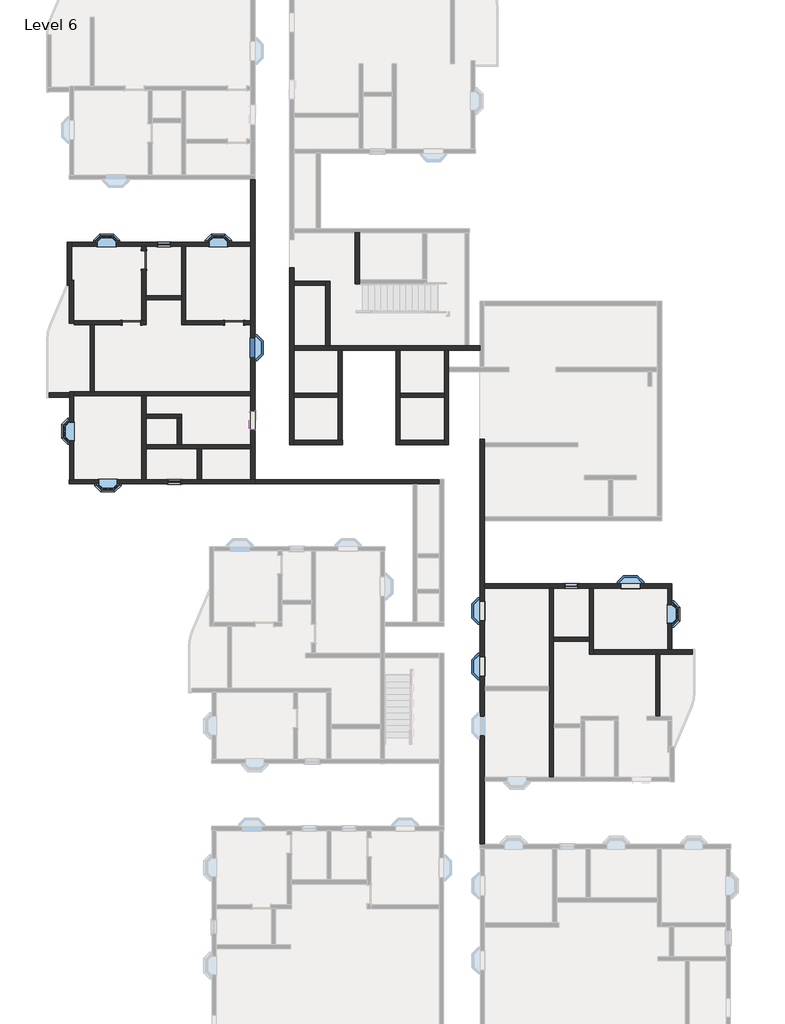
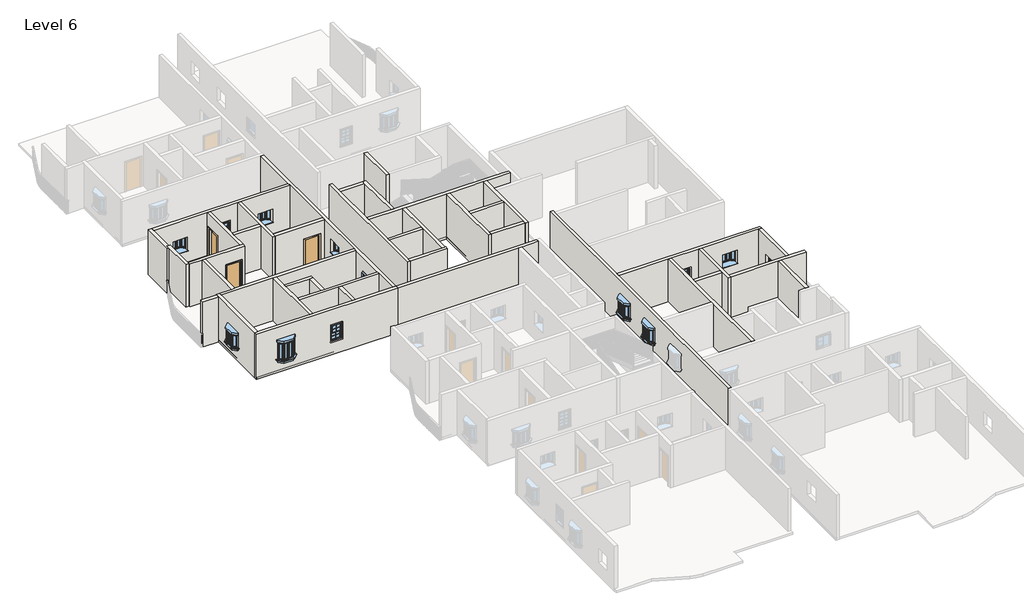
# One storey, part 3 of 14: 40 walls, 13 windows, 3 doors.
# Revit data of these elements (continued)
# Element 26 (IfcWall, "9\"")
#   Top Offset = 0' - 0"
#   Base Offset = 0' - 0"
#   wall height = 10' - 0"
#   Phase Created = New Construction
#   Base Constraint = Level 6
#   Top Constraint = Level 7
#   Materials on its faces: "Earth", "Default Wall"
# Element 27 (IfcWall, "9\"")
#   Top Offset = 0' - 0"
#   Base Offset = 0' - 0"
#   wall height = 10' - 0"
#   Phase Created = New Construction
#   Base Constraint = Level 6
#   Top Constraint = Level 7
#   Materials on its faces: "Default Wall", "Default Mass Interior Wall"
# Element 28 (IfcWall, "9\"")
#   Top Offset = 0' - 0"
#   Base Offset = 0' - 0"
#   wall height = 10' - 0"
#   Phase Created = New Construction
#   Base Constraint = Level 6
#   Top Constraint = Level 7
#   Materials on its faces: "Default Wall"
# Element 29 (IfcWall, "9\"")
#   Top Offset = 0' - 0"
#   Base Offset = 0' - 0"
#   wall height = 10' - 0"
#   Phase Created = New Construction
#   Base Constraint = Level 6
#   Top Constraint = Level 7
#   Materials on its faces: "Default Wall", "Default Mass Interior Wall", "Earth"
# Elements 30, 33, 34, 35, 36, 37, 38, 39, 40, 41 (IfcWall, "9\" w")
#   Top Offset = 0' - 0"
#   Base Offset = 0' - 0"
#   wall height = 10' - 0"
#   Phase Created = New Construction
#   Base Constraint = Level 6
#   Top Constraint = Level 7
#   Materials on its faces: "Default Wall"
# Element 31 (IfcWall, "9\" w")
#   Top Offset = 0' - 0"
#   Base Offset = 0' - 0"
#   wall height = 10' - 0"
#   Phase Created = New Construction
#   Base Constraint = Level 6
#   Top Constraint = Level 7
#   Materials on its faces: "Default Wall", "Earth"
# Element 32 (IfcWall, "9\" w")
#   Top Offset = 0' - 0"
#   Base Offset = 0' - 0"
#   wall height = 10' - 0"
#   Phase Created = New Construction
#   Base Constraint = Level 6
#   Top Constraint = Level 7
#   Materials on its faces: "Default Wall", "Brick, Soldier Course"
# Element 42 (IfcWall, "9\" w")
#   Top Offset = 0' - 0"
#   Base Offset = 0' - 0"
#   wall height = 10' - 0"
#   Phase Created = New Construction
#   Base Constraint = Level 6
#   Top Constraint = Level 7
#   Materials on its faces: "Default Wall", "Wood - Stained"
# Element 43 (IfcWall, "9\" w")
#   Top Offset = 0' - 0"
#   Base Offset = 0' - 0"
#   wall height = 10' - 0"
#   Phase Created = New Construction
#   Base Constraint = Level 6
#   Top Constraint = Level 7
#   Materials on its faces: "Default Wall", "Acoustic Ceiling Tile 24 x 24"
# Element 44 (IfcWindow, "910x1210mm")
#   Mark = "361"
#   Phase Created = New Construction
#   Materials on its faces: "Window Frame", "Glass"
# Element 45 (IfcWindow, "910x910mm")
#   Mark = "337"
#   Phase Created = New Construction
#   Materials on its faces: "Window Frame", "Glass"
# Element 46 (IfcWindow, "910x910mm")
#   Mark = "338"
#   Phase Created = New Construction
#   Materials on its faces: "Window Frame", "Glass"
# Element 47 (IfcWindow, "910x910mm")
#   Mark = "310"
#   Phase Created = New Construction
#   Materials on its faces: "Window Frame", "Glass"
# Element 48 (IfcWindow, "910x910mm")
#   Mark = "311"
#   Phase Created = New Construction
#   Materials on its faces: "Window Frame", "Glass"
# Element 49 (IfcWindow, "910x910mm")
#   Mark = "312"
#   Phase Created = New Construction
#   Materials on its faces: "Window Frame", "Glass"
# Element 50 (IfcWindow, "910x910mm")
#   Mark = "313"
#   Phase Created = New Construction
#   Materials on its faces: "Window Frame", "Glass"
# Element 51 (IfcWindow, "910x910mm")
#   Mark = "335"
#   Phase Created = New Construction
#   Materials on its faces: "Window Frame", "Glass"
# Element 52 (IfcWindow, "910x910mm")
#   Mark = "336"
#   Phase Created = New Construction
#   Materials on its faces: "Window Frame", "Glass"
# Element 53 (IfcWindow, "Window-Double-Hung : 26\" x 42\"")
#   Mark = "359"
#   Window Inset = 0' - 0"
#   Interior Wall Closure = 0' - 1 1/2"
#   Frame Extension = 0' - 1 1/4"
#   Exterior Wall Closure = 0' - 0 1/2"
#   Interior Trim Visibility = yes
#   Indicator Visibility = yes
#   Exterior Trim Visibility = yes
#   Phase Created = New Construction
#   Materials on its faces: "Wood - Stained", "Glass", "Clad - White"
# Element 54 (IfcWindow, "Window-Double-Hung : 26\" x 42\"")
#   Mark = "348"
#   Window Inset = 0' - 0"
#   Interior Wall Closure = 0' - 1 1/2"
#   Frame Extension = 0' - 1 1/4"
#   Exterior Wall Closure = 0' - 0 1/2"
#   Interior Trim Visibility = yes
#   Indicator Visibility = yes
#   Exterior Trim Visibility = yes
#   Phase Created = New Construction
#   Materials on its faces: "Wood - Stained", "Glass", "Clad - White"
# Element 55 (IfcWindow, "Window-Double-Hung : 26\" x 42\"")
#   Mark = "349"
#   Window Inset = 0' - 0"
#   Interior Wall Closure = 0' - 1 1/2"
#   Frame Extension = 0' - 1 1/4"
#   Exterior Wall Closure = 0' - 0 1/2"
#   Interior Trim Visibility = yes
#   Indicator Visibility = yes
#   Exterior Trim Visibility = yes
#   Phase Created = New Construction
#   Materials on its faces: "Wood - Stained", "Glass", "Clad - White"
# Element 56 (IfcWindow, "Windows_Sgl_w-Glazing_Bars : 910x910mm")
#   Mark = "344"
#   Phase Created = New Construction
#   Materials on its faces: "Window Frame", "Glass"
# Materials
#   "Door - Panel": class "Wood", colour RGB 210 159 95, transparency 0, Cost = 0
#   "Door - Frame": colour RGB 118 70 51, transparency 0, Cost = 0
#   "Window Frame": colour RGB 249 249 249, transparency 0
#   "Glass": class "Glass", colour RGB 0 128 192, transparency 0.75, Description = "Soda Lime Glass", Cost = 0
#   "Wood - Stained": class "Wood", colour RGB 224 178 126, transparency 0, Cost = 0
#   "Clad - White": class "Wood", colour RGB 242 242 238, transparency 0, Cost = 0
#   "Default Wall": colour RGB 128 128 128, transparency 0, Cost = 0
#   "Cherry": class "Wood", colour RGB 226 177 128, transparency 0, Description = "Prunus Serotina", Cost = 0
#   "Parking Stripe": class "Paint", colour RGB 250 250 91, transparency 0, Cost = 0
#   "Earth": class "Generic", colour RGB 97 75 62, transparency 0, Description = "Soil", Cost = 0
#   "Default Mass Interior Wall": class "Generic", colour RGB 195 229 126, transparency 0, Cost = 0
#   "Brick, Soldier Course": class "Masonry", colour RGB 170 98 104, transparency 0, Description = "Common brick soldier coursed", Cost = 0
#   "Acoustic Ceiling Tile 24 x 24": class "Generic", colour RGB 232 232 232, transparency 0, Description = "Acoustic Ceiling Tile 24 x 24", Cost = 0
